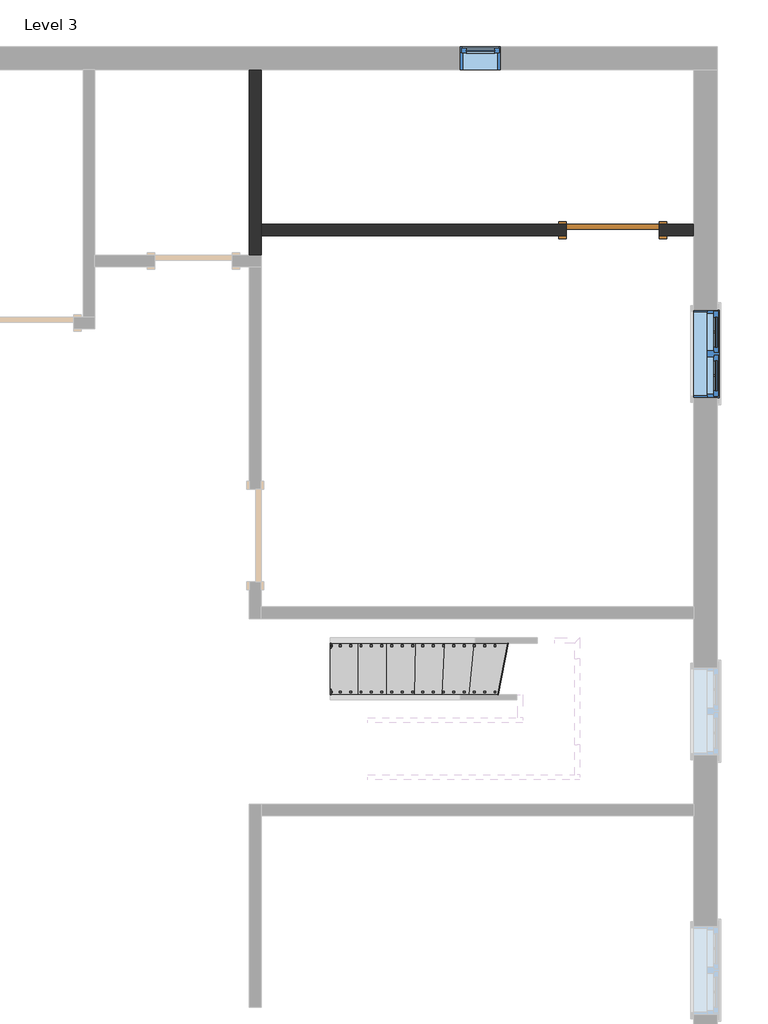
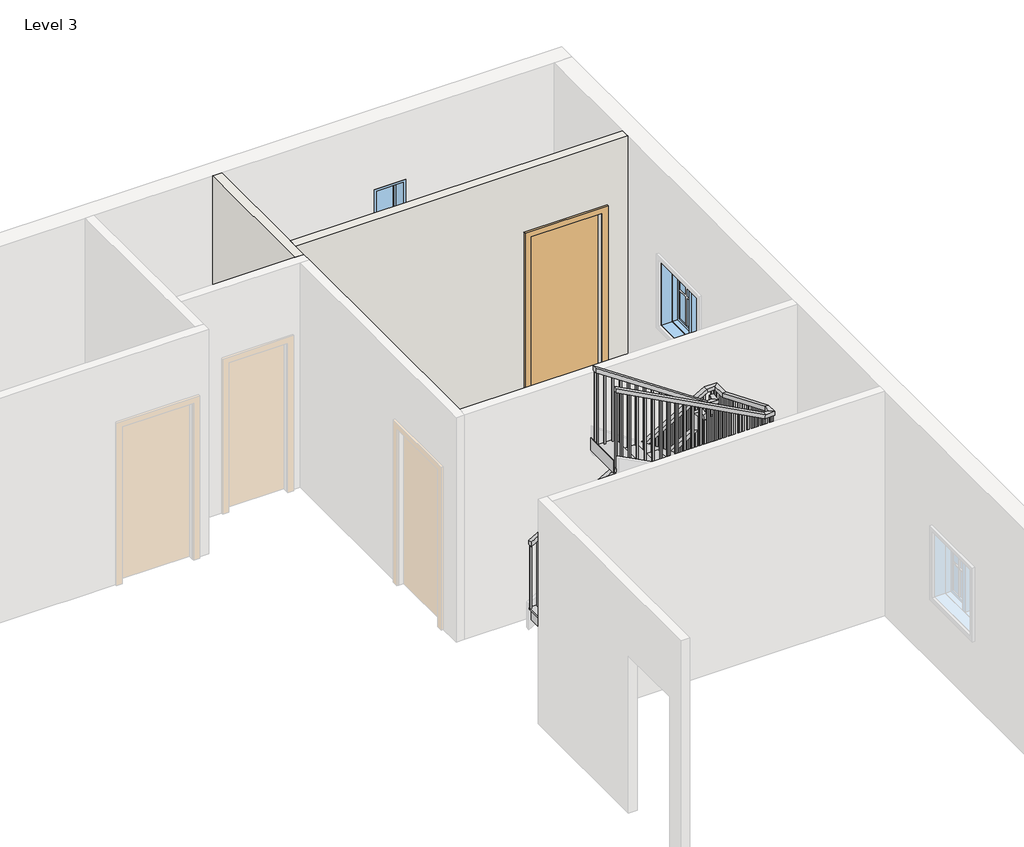
# One storey, part 2 of 3: 2 railings, 2 walls, 2 windows, 1 door, 1 stair flight.
"""IFC4 building model written with IfcOpenShell, lengths in millimetres."""

from ifc_helpers import new_model, si_unit, frame, origin, place, context, project, spatial, polyline, outline, extrude, faceted_brep, transform, mapped, element, save
from components import door_e5f9f3c4, stair_flight_4e66bfb9, window_373d1f99, window_339605e1

model = new_model("IFC4")

# Units and contexts
model_context = context("Model", 3, world=origin())
ifc_project = project(units=[si_unit("LENGTHUNIT", "METRE", prefix="MILLI")], contexts=[model_context])

# Site, building, storey
site = spatial("IfcSite", under=ifc_project)
building = spatial("IfcBuilding", under=site)
storey = spatial("IfcBuildingStorey", under=building, Name="Level 3", Elevation=3200.4)

# Door
placement = place(None, origin())
door_shape = door_e5f9f3c4(model_context)
element("IfcDoor", 1, ObjectType="Single-Flush : 36\" x 84\"", at=placement, inside=storey, context=model_context, shape_type="MappedRepresentation", body=[
    mapped(door_shape, transform((3624.6756993, 7272.227558, 3200.4), x_axis=(1.0, 0.0, 0.0), y_axis=(0.0, 1.0, 0.0), z_axis=(0.0, 0.0, 1.0))),
])

# Railings
element("IfcRailing", 2, ObjectType="Handrail - Rectangular", at=placement, inside=storey, context=model_context, shape_type="SolidModel", body=[
    faceted_brep([(838.4202681, 2744.677558, 4453.4666667), (838.4202681, 2744.677558, 4393.1442501), (838.4202681, 2693.877558, 4393.1442501), (838.4202681, 2693.877558, 4453.4666667), (2663.2073911, 2744.677558, 5621.9510761), (2714.0073911, 2744.677558, 5594.1579377), (2714.0073911, 2693.877558, 5594.1579377), (2663.2073911, 2693.877558, 5621.9510761), (2663.2073911, 2744.677558, 5834.2070819), (2714.0073911, 2744.677558, 5783.4070819), (2714.0073911, 2693.877558, 5783.4070819), (2663.2073911, 2693.877558, 5834.2070819), (2790.2073911, 2744.677558, 5834.2070819), (2790.2073911, 2744.677558, 5783.4070819), (2739.4073911, 2693.877558, 5783.4070819), (2739.4073911, 2693.877558, 5834.2070819), (2790.2073911, 2617.677558, 5834.2070819), (2790.2073911, 2595.5706127, 5783.4070819), (2739.4073911, 2595.5706127, 5783.4070819), (2739.4073911, 2617.677558, 5834.2070819), (2790.2073911, 2490.677558, 5970.5650362), (2790.2073911, 2439.877558, 5950.5723294), (2739.4073911, 2439.877558, 5950.5723294), (2739.4073911, 2490.677558, 5970.5650362), (2790.2073911, 2490.677558, 6186.1137911), (2790.2073911, 2439.877558, 6135.3137911), (2739.4073911, 2439.877558, 6135.3137911), (2739.4073911, 2490.677558, 6186.1137911), (2790.2073911, 2363.677558, 6186.1137911), (2790.2073911, 2363.677558, 6135.3137911), (2739.4073911, 2414.477558, 6135.3137911), (2739.4073911, 2414.477558, 6186.1137911), (2663.2073911, 2363.677558, 6186.1137911), (2647.7076469, 2363.677558, 6135.3137911), (2647.7076469, 2414.477558, 6135.3137911), (2663.2073911, 2414.477558, 6186.1137911), (1211.6756993, 2363.677558, 7162.8), (1211.6756993, 2414.477558, 7162.8), (1211.6756993, 2414.477558, 7101.5707504), (1211.6756993, 2363.677558, 7101.5707504)], [[[0, 1, 2, 3]], [[1, 0, 4, 5]], [[2, 1, 5, 6]], [[3, 2, 6, 7]], [[0, 3, 7, 4]], [[5, 4, 8, 9]], [[6, 5, 9, 10]], [[7, 6, 10, 11]], [[4, 7, 11, 8]], [[9, 8, 12, 13]], [[10, 9, 13, 14]], [[11, 10, 14, 15]], [[8, 11, 15, 12]], [[13, 12, 16, 17]], [[14, 13, 17, 18]], [[15, 14, 18, 19]], [[12, 15, 19, 16]], [[17, 16, 20, 21]], [[18, 17, 21, 22]], [[19, 18, 22, 23]], [[16, 19, 23, 20]], [[21, 20, 24, 25]], [[22, 21, 25, 26]], [[23, 22, 26, 27]], [[20, 23, 27, 24]], [[25, 24, 28, 29]], [[26, 25, 29, 30]], [[27, 26, 30, 31]], [[24, 27, 31, 28]], [[29, 28, 32, 33]], [[30, 29, 33, 34]], [[31, 30, 34, 35]], [[28, 31, 35, 32]], [[36, 37, 38, 39]], [[33, 32, 36, 39]], [[34, 33, 39, 38]], [[35, 34, 38, 37]], [[32, 35, 37, 36]]]),
    extrude(outline(polyline([(7075.5599798, 1250.3323911), (7088.3780756, 1231.2823911), (6079.0666667, 1231.2823911), (6079.0666667, 1250.3323911), (7075.5599798, 1250.3323911)])), frame((0.0, 2379.552558, 0.0), z_axis=(0.0, 1.0, 0.0), x_axis=(0.0, 0.0, 1.0)), (0.0, 0.0, 1.0), 19.05),
    extrude(outline(polyline([(7007.1968022, 1351.9323911), (7020.014898, 1332.8823911), (6079.0666667, 1332.8823911), (6079.0666667, 1351.9323911), (7007.1968022, 1351.9323911)])), frame((0.0, 2379.552558, 0.0), z_axis=(0.0, 1.0, 0.0), x_axis=(0.0, 0.0, 1.0)), (0.0, 0.0, 1.0), 19.05),
    extrude(outline(polyline([(6938.8336246, 1453.5323911), (6951.6517204, 1434.4823911), (6079.0666667, 1434.4823911), (6079.0666667, 1453.5323911), (6938.8336246, 1453.5323911)])), frame((0.0, 2379.552558, 0.0), z_axis=(0.0, 1.0, 0.0), x_axis=(0.0, 0.0, 1.0)), (0.0, 0.0, 1.0), 19.05),
    extrude(outline(polyline([(6870.470447, 1555.1323911), (6883.2885428, 1536.0823911), (5909.7333333, 1536.0823911), (5909.7333333, 1555.1323911), (6870.470447, 1555.1323911)])), frame((0.0, 2379.552558, 0.0), z_axis=(0.0, 1.0, 0.0), x_axis=(0.0, 0.0, 1.0)), (0.0, 0.0, 1.0), 19.05),
    extrude(outline(polyline([(6802.1072694, 1656.7323911), (6814.9253652, 1637.6823911), (5909.7333333, 1637.6823911), (5909.7333333, 1656.7323911), (6802.1072694, 1656.7323911)])), frame((0.0, 2379.552558, 0.0), z_axis=(0.0, 1.0, 0.0), x_axis=(0.0, 0.0, 1.0)), (0.0, 0.0, 1.0), 19.05),
    extrude(outline(polyline([(6733.7440918, 1758.3323911), (6746.5621876, 1739.2823911), (5909.7333333, 1739.2823911), (5909.7333333, 1758.3323911), (6733.7440918, 1758.3323911)])), frame((0.0, 2379.552558, 0.0), z_axis=(0.0, 1.0, 0.0), x_axis=(0.0, 0.0, 1.0)), (0.0, 0.0, 1.0), 19.05),
    extrude(outline(polyline([(6665.3809143, 1859.9323911), (6678.1990101, 1840.8823911), (5740.4, 1840.8823911), (5740.4, 1859.9323911), (6665.3809143, 1859.9323911)])), frame((0.0, 2379.552558, 0.0), z_axis=(0.0, 1.0, 0.0), x_axis=(0.0, 0.0, 1.0)), (0.0, 0.0, 1.0), 19.05),
    extrude(outline(polyline([(6597.0177367, 1961.5323911), (6609.8358325, 1942.4823911), (5740.4, 1942.4823911), (5740.4, 1961.5323911), (6597.0177367, 1961.5323911)])), frame((0.0, 2379.552558, 0.0), z_axis=(0.0, 1.0, 0.0), x_axis=(0.0, 0.0, 1.0)), (0.0, 0.0, 1.0), 19.05),
    extrude(outline(polyline([(6528.6545591, 2063.1323911), (6541.4726549, 2044.0823911), (5571.0666667, 2044.0823911), (5571.0666667, 2063.1323911), (6528.6545591, 2063.1323911)])), frame((0.0, 2379.552558, 0.0), z_axis=(0.0, 1.0, 0.0), x_axis=(0.0, 0.0, 1.0)), (0.0, 0.0, 1.0), 19.05),
    extrude(outline(polyline([(6460.2913815, 2164.7323911), (6473.1094773, 2145.6823911), (5571.0666667, 2145.6823911), (5571.0666667, 2164.7323911), (6460.2913815, 2164.7323911)])), frame((0.0, 2379.552558, 0.0), z_axis=(0.0, 1.0, 0.0), x_axis=(0.0, 0.0, 1.0)), (0.0, 0.0, 1.0), 19.05),
    extrude(outline(polyline([(6391.9282039, 2266.3323911), (6404.7462997, 2247.2823911), (5571.0666667, 2247.2823911), (5571.0666667, 2266.3323911), (6391.9282039, 2266.3323911)])), frame((0.0, 2379.552558, 0.0), z_axis=(0.0, 1.0, 0.0), x_axis=(0.0, 0.0, 1.0)), (0.0, 0.0, 1.0), 19.05),
    extrude(outline(polyline([(6323.5650263, 2367.9323911), (6336.3831221, 2348.8823911), (5401.7333333, 2348.8823911), (5401.7333333, 2367.9323911), (6323.5650263, 2367.9323911)])), frame((0.0, 2379.552558, 0.0), z_axis=(0.0, 1.0, 0.0), x_axis=(0.0, 0.0, 1.0)), (0.0, 0.0, 1.0), 19.05),
    extrude(outline(polyline([(6255.2018487, 2469.5323911), (6268.0199445, 2450.4823911), (5401.7333333, 2450.4823911), (5401.7333333, 2469.5323911), (6255.2018487, 2469.5323911)])), frame((0.0, 2379.552558, 0.0), z_axis=(0.0, 1.0, 0.0), x_axis=(0.0, 0.0, 1.0)), (0.0, 0.0, 1.0), 19.05),
    extrude(outline(polyline([(6186.8386712, 2571.1323911), (6199.656767, 2552.0823911), (5232.4, 2552.0823911), (5232.4, 2571.1323911), (6186.8386712, 2571.1323911)])), frame((0.0, 2379.552558, 0.0), z_axis=(0.0, 1.0, 0.0), x_axis=(0.0, 0.0, 1.0)), (0.0, 0.0, 1.0), 19.05),
    extrude(outline(polyline([(6118.4754936, 2672.7323911), (6131.2935894, 2653.6823911), (5232.4, 2653.6823911), (5232.4, 2672.7323911), (6118.4754936, 2672.7323911)])), frame((0.0, 2379.552558, 0.0), z_axis=(0.0, 1.0, 0.0), x_axis=(0.0, 0.0, 1.0)), (0.0, 0.0, 1.0), 19.05),
    extrude(outline(polyline([(2755.2823911, 2424.002558), (2774.3323911, 2424.002558), (2774.3323911, 2404.952558), (2755.2823911, 2404.952558), (2755.2823911, 2424.002558)])), frame((0.0, 0.0, 5063.0666667), z_axis=(0.0, 0.0, 1.0), x_axis=(1.0, 0.0, 0.0)), (0.0, 0.0, 1.0), 1072.2471245),
    extrude(outline(polyline([(2506.552558, 5878.9844034), (2525.602558, 5858.5307103), (2525.602558, 4893.7333333), (2506.552558, 4893.7333333), (2506.552558, 5878.9844034)])), frame((2755.2823911, 0.0, 0.0), z_axis=(1.0, 0.0, 0.0), x_axis=(0.0, 1.0, 0.0)), (0.0, 0.0, 1.0), 19.05),
    extrude(outline(polyline([(2608.152558, 5769.89804), (2627.202558, 5749.4443468), (2627.202558, 4893.7333333), (2608.152558, 4893.7333333), (2608.152558, 5769.89804)])), frame((2755.2823911, 0.0, 0.0), z_axis=(1.0, 0.0, 0.0), x_axis=(0.0, 1.0, 0.0)), (0.0, 0.0, 1.0), 19.05),
    extrude(outline(polyline([(2657.6952681, 2709.752558), (2657.6952681, 2728.802558), (2676.7452681, 2728.802558), (2676.7452681, 2709.752558), (2657.6952681, 2709.752558)])), frame((0.0, 0.0, 4555.0666667), z_axis=(0.0, 0.0, 1.0), x_axis=(1.0, 0.0, 0.0)), (0.0, 0.0, 1.0), 1228.3404152),
    extrude(outline(polyline([(5505.2389489, 2575.1452681), (5493.0404695, 2556.0952681), (4555.0666667, 2556.0952681), (4555.0666667, 2575.1452681), (5505.2389489, 2575.1452681)])), frame((0.0, 2709.752558, 0.0), z_axis=(0.0, 1.0, 0.0), x_axis=(0.0, 0.0, 1.0)), (0.0, 0.0, 1.0), 19.05),
    extrude(outline(polyline([(5440.1803925, 2473.5452681), (5427.9819131, 2454.4952681), (4385.7333333, 2454.4952681), (4385.7333333, 2473.5452681), (5440.1803925, 2473.5452681)])), frame((0.0, 2709.752558, 0.0), z_axis=(0.0, 1.0, 0.0), x_axis=(0.0, 0.0, 1.0)), (0.0, 0.0, 1.0), 19.05),
    extrude(outline(polyline([(5375.121836, 2371.9452681), (5362.9233567, 2352.8952681), (4385.7333333, 2352.8952681), (4385.7333333, 2371.9452681), (5375.121836, 2371.9452681)])), frame((0.0, 2709.752558, 0.0), z_axis=(0.0, 1.0, 0.0), x_axis=(0.0, 0.0, 1.0)), (0.0, 0.0, 1.0), 19.05),
    extrude(outline(polyline([(5310.0632796, 2270.3452681), (5297.8648003, 2251.2952681), (4385.7333333, 2251.2952681), (4385.7333333, 2270.3452681), (5310.0632796, 2270.3452681)])), frame((0.0, 2709.752558, 0.0), z_axis=(0.0, 1.0, 0.0), x_axis=(0.0, 0.0, 1.0)), (0.0, 0.0, 1.0), 19.05),
    extrude(outline(polyline([(5245.0047232, 2168.7452681), (5232.8062439, 2149.6952681), (4216.4, 2149.6952681), (4216.4, 2168.7452681), (5245.0047232, 2168.7452681)])), frame((0.0, 2709.752558, 0.0), z_axis=(0.0, 1.0, 0.0), x_axis=(0.0, 0.0, 1.0)), (0.0, 0.0, 1.0), 19.05),
    extrude(outline(polyline([(5179.9461668, 2067.1452681), (5167.7476875, 2048.0952681), (4216.4, 2048.0952681), (4216.4, 2067.1452681), (5179.9461668, 2067.1452681)])), frame((0.0, 2709.752558, 0.0), z_axis=(0.0, 1.0, 0.0), x_axis=(0.0, 0.0, 1.0)), (0.0, 0.0, 1.0), 19.05),
    extrude(outline(polyline([(5114.8876104, 1965.5452681), (5102.689131, 1946.4952681), (4216.4, 1946.4952681), (4216.4, 1965.5452681), (5114.8876104, 1965.5452681)])), frame((0.0, 2709.752558, 0.0), z_axis=(0.0, 1.0, 0.0), x_axis=(0.0, 0.0, 1.0)), (0.0, 0.0, 1.0), 19.05),
    extrude(outline(polyline([(5049.8290539, 1863.9452681), (5037.6305746, 1844.8952681), (4047.0666667, 1844.8952681), (4047.0666667, 1863.9452681), (5049.8290539, 1863.9452681)])), frame((0.0, 2709.752558, 0.0), z_axis=(0.0, 1.0, 0.0), x_axis=(0.0, 0.0, 1.0)), (0.0, 0.0, 1.0), 19.05),
    extrude(outline(polyline([(4984.7704975, 1762.3452681), (4972.5720182, 1743.2952681), (4047.0666667, 1743.2952681), (4047.0666667, 1762.3452681), (4984.7704975, 1762.3452681)])), frame((0.0, 2709.752558, 0.0), z_axis=(0.0, 1.0, 0.0), x_axis=(0.0, 0.0, 1.0)), (0.0, 0.0, 1.0), 19.05),
    extrude(outline(polyline([(4919.7119411, 1660.7452681), (4907.5134618, 1641.6952681), (3877.7333333, 1641.6952681), (3877.7333333, 1660.7452681), (4919.7119411, 1660.7452681)])), frame((0.0, 2709.752558, 0.0), z_axis=(0.0, 1.0, 0.0), x_axis=(0.0, 0.0, 1.0)), (0.0, 0.0, 1.0), 19.05),
    extrude(outline(polyline([(4854.6533847, 1559.1452681), (4842.4549054, 1540.0952681), (3877.7333333, 1540.0952681), (3877.7333333, 1559.1452681), (4854.6533847, 1559.1452681)])), frame((0.0, 2709.752558, 0.0), z_axis=(0.0, 1.0, 0.0), x_axis=(0.0, 0.0, 1.0)), (0.0, 0.0, 1.0), 19.05),
    extrude(outline(polyline([(4789.5948283, 1457.5452681), (4777.3963489, 1438.4952681), (3877.7333333, 1438.4952681), (3877.7333333, 1457.5452681), (4789.5948283, 1457.5452681)])), frame((0.0, 2709.752558, 0.0), z_axis=(0.0, 1.0, 0.0), x_axis=(0.0, 0.0, 1.0)), (0.0, 0.0, 1.0), 19.05),
    extrude(outline(polyline([(4724.5362719, 1355.9452681), (4712.3377925, 1336.8952681), (3708.4, 1336.8952681), (3708.4, 1355.9452681), (4724.5362719, 1355.9452681)])), frame((0.0, 2709.752558, 0.0), z_axis=(0.0, 1.0, 0.0), x_axis=(0.0, 0.0, 1.0)), (0.0, 0.0, 1.0), 19.05),
    extrude(outline(polyline([(4659.4777154, 1254.3452681), (4647.2792361, 1235.2952681), (3708.4, 1235.2952681), (3708.4, 1254.3452681), (4659.4777154, 1254.3452681)])), frame((0.0, 2709.752558, 0.0), z_axis=(0.0, 1.0, 0.0), x_axis=(0.0, 0.0, 1.0)), (0.0, 0.0, 1.0), 19.05),
    extrude(outline(polyline([(4594.419159, 1152.7452681), (4582.2206797, 1133.6952681), (3708.4, 1133.6952681), (3708.4, 1152.7452681), (4594.419159, 1152.7452681)])), frame((0.0, 2709.752558, 0.0), z_axis=(0.0, 1.0, 0.0), x_axis=(0.0, 0.0, 1.0)), (0.0, 0.0, 1.0), 19.05),
    extrude(outline(polyline([(4529.3606026, 1051.1452681), (4517.1621233, 1032.0952681), (3539.0666667, 1032.0952681), (3539.0666667, 1051.1452681), (4529.3606026, 1051.1452681)])), frame((0.0, 2709.752558, 0.0), z_axis=(0.0, 1.0, 0.0), x_axis=(0.0, 0.0, 1.0)), (0.0, 0.0, 1.0), 19.05),
    extrude(outline(polyline([(4464.3020462, 949.5452681), (4452.1035669, 930.4952681), (3539.0666667, 930.4952681), (3539.0666667, 949.5452681), (4464.3020462, 949.5452681)])), frame((0.0, 2709.752558, 0.0), z_axis=(0.0, 1.0, 0.0), x_axis=(0.0, 0.0, 1.0)), (0.0, 0.0, 1.0), 19.05),
    extrude(outline(polyline([(2755.2823911, 2398.602558), (2774.3323911, 2398.602558), (2774.3323911, 2379.552558), (2755.2823911, 2379.552558), (2755.2823911, 2398.602558)])), frame((0.0, 0.0, 5063.0666667), z_axis=(0.0, 0.0, 1.0), x_axis=(1.0, 0.0, 0.0)), (0.0, 0.0, 1.0), 1072.2471245),
    extrude(outline(polyline([(2755.2823911, 2709.752558), (2755.2823911, 2728.802558), (2774.3323911, 2728.802558), (2774.3323911, 2709.752558), (2755.2823911, 2709.752558)])), frame((0.0, 0.0, 4724.4), z_axis=(0.0, 0.0, 1.0), x_axis=(1.0, 0.0, 0.0)), (0.0, 0.0, 1.0), 1059.0070819),
    extrude(outline(polyline([(7088.7526546, 1230.7256993), (7101.5707504, 1211.6756993), (6079.0666667, 1211.6756993), (6079.0666667, 1230.7256993), (7088.7526546, 1230.7256993)])), frame((0.0, 2379.552558, 0.0), z_axis=(0.0, 1.0, 0.0), x_axis=(0.0, 0.0, 1.0)), (0.0, 0.0, 1.0), 19.05),
    extrude(outline(polyline([(4405.3427294, 857.4702681), (4393.1442501, 838.4202681), (3539.0666667, 838.4202681), (3539.0666667, 857.4702681), (4405.3427294, 857.4702681)])), frame((0.0, 2709.752558, 0.0), z_axis=(0.0, 1.0, 0.0), x_axis=(0.0, 0.0, 1.0)), (0.0, 0.0, 1.0), 19.05),
])
element("IfcRailing", 3, ObjectType="Handrail - Rectangular", at=placement, inside=storey, context=model_context, shape_type="SolidModel", body=[
    faceted_brep([(838.4202681, 3202.4524989, 4453.4666667), (838.4202681, 3202.4524989, 4394.8953096), (838.4202681, 3151.6524989, 4394.8953096), (838.4202681, 3151.6524989, 4453.4666667), (3089.9785641, 3202.4524989, 5745.6368493), (3103.5198636, 3202.4524989, 5694.8368493), (3103.5198636, 3151.6524989, 5694.8368493), (3089.9785641, 3151.6524989, 5745.6368493), (3247.982332, 3202.4524989, 5745.6368493), (3247.982332, 3202.4524989, 5694.8368493), (3197.182332, 3151.6524989, 5694.8368493), (3197.182332, 3151.6524989, 5745.6368493), (3247.982332, 2995.1725832, 5745.6368493), (3247.982332, 2984.9732412, 5694.8368493), (3197.182332, 2984.9732412, 5694.8368493), (3197.182332, 2995.1725832, 5745.6368493), (3247.982332, 2050.6126885, 6140.8552365), (3247.982332, 2040.4133465, 6090.0552365), (3197.182332, 2040.4133465, 6090.0552365), (3197.182332, 2050.6126885, 6140.8552365), (3247.982332, 1905.9026171, 6140.8552365), (3247.982332, 1905.9026171, 6090.0552365), (3197.182332, 1956.7026171, 6090.0552365), (3197.182332, 1956.7026171, 6140.8552365), (3128.9262072, 1905.9026171, 6140.8552365), (3116.2326609, 1905.9026171, 6090.0552365), (3116.2326609, 1956.7026171, 6090.0552365), (3128.9262072, 1956.7026171, 6140.8552365), (1211.6756993, 1905.9026171, 7162.8), (1211.6756993, 1956.7026171, 7162.8), (1211.6756993, 1956.7026171, 7105.2340072), (1211.6756993, 1905.9026171, 7105.2340072)], [[[0, 1, 2, 3]], [[1, 0, 4, 5]], [[2, 1, 5, 6]], [[3, 2, 6, 7]], [[0, 3, 7, 4]], [[5, 4, 8, 9]], [[6, 5, 9, 10]], [[7, 6, 10, 11]], [[4, 7, 11, 8]], [[9, 8, 12, 13]], [[10, 9, 13, 14]], [[11, 10, 14, 15]], [[8, 11, 15, 12]], [[13, 12, 16, 17]], [[14, 13, 17, 18]], [[15, 14, 18, 19]], [[12, 15, 19, 16]], [[17, 16, 20, 21]], [[18, 17, 21, 22]], [[19, 18, 22, 23]], [[16, 19, 23, 20]], [[21, 20, 24, 25]], [[22, 21, 25, 26]], [[23, 22, 26, 27]], [[20, 23, 27, 24]], [[28, 29, 30, 31]], [[25, 24, 28, 31]], [[26, 25, 31, 30]], [[27, 26, 30, 29]], [[24, 27, 29, 28]]]),
    extrude(outline(polyline([(7067.3989368, 1282.657332), (6079.0666667, 1282.657332), (6079.0666667, 1301.707332), (7057.2447876, 1301.707332), (7067.3989368, 1282.657332)])), frame((0.0, 1921.7776171, 0.0), z_axis=(0.0, 1.0, 0.0), x_axis=(0.0, 0.0, 1.0)), (0.0, 0.0, 1.0), 19.05),
    extrude(outline(polyline([(7013.2434743, 1384.257332), (6079.0666667, 1384.257332), (6079.0666667, 1403.307332), (7003.0893251, 1403.307332), (7013.2434743, 1384.257332)])), frame((0.0, 1921.7776171, 0.0), z_axis=(0.0, 1.0, 0.0), x_axis=(0.0, 0.0, 1.0)), (0.0, 0.0, 1.0), 19.05),
    extrude(outline(polyline([(6959.0880118, 1485.857332), (5909.7333333, 1485.857332), (5909.7333333, 1504.907332), (6948.9338626, 1504.907332), (6959.0880118, 1485.857332)])), frame((0.0, 1921.7776171, 0.0), z_axis=(0.0, 1.0, 0.0), x_axis=(0.0, 0.0, 1.0)), (0.0, 0.0, 1.0), 19.05),
    extrude(outline(polyline([(6904.9325493, 1587.457332), (5909.7333333, 1587.457332), (5909.7333333, 1606.507332), (6894.7784001, 1606.507332), (6904.9325493, 1587.457332)])), frame((0.0, 1921.7776171, 0.0), z_axis=(0.0, 1.0, 0.0), x_axis=(0.0, 0.0, 1.0)), (0.0, 0.0, 1.0), 19.05),
    extrude(outline(polyline([(6850.7770868, 1689.057332), (5909.7333333, 1689.057332), (5909.7333333, 1708.107332), (6840.6229376, 1708.107332), (6850.7770868, 1689.057332)])), frame((0.0, 1921.7776171, 0.0), z_axis=(0.0, 1.0, 0.0), x_axis=(0.0, 0.0, 1.0)), (0.0, 0.0, 1.0), 19.05),
    extrude(outline(polyline([(6796.6216243, 1790.657332), (5740.4, 1790.657332), (5740.4, 1809.707332), (6786.4674751, 1809.707332), (6796.6216243, 1790.657332)])), frame((0.0, 1921.7776171, 0.0), z_axis=(0.0, 1.0, 0.0), x_axis=(0.0, 0.0, 1.0)), (0.0, 0.0, 1.0), 19.05),
    extrude(outline(polyline([(6742.4661618, 1892.257332), (5740.4, 1892.257332), (5740.4, 1911.307332), (6732.3120126, 1911.307332), (6742.4661618, 1892.257332)])), frame((0.0, 1921.7776171, 0.0), z_axis=(0.0, 1.0, 0.0), x_axis=(0.0, 0.0, 1.0)), (0.0, 0.0, 1.0), 19.05),
    extrude(outline(polyline([(6688.3106993, 1993.857332), (5740.4, 1993.857332), (5740.4, 2012.907332), (6678.1565501, 2012.907332), (6688.3106993, 1993.857332)])), frame((0.0, 1921.7776171, 0.0), z_axis=(0.0, 1.0, 0.0), x_axis=(0.0, 0.0, 1.0)), (0.0, 0.0, 1.0), 19.05),
    extrude(outline(polyline([(6634.1552369, 2095.457332), (5571.0666667, 2095.457332), (5571.0666667, 2114.507332), (6624.0010876, 2114.507332), (6634.1552369, 2095.457332)])), frame((0.0, 1921.7776171, 0.0), z_axis=(0.0, 1.0, 0.0), x_axis=(0.0, 0.0, 1.0)), (0.0, 0.0, 1.0), 19.05),
    extrude(outline(polyline([(6579.9997744, 2197.057332), (5571.0666667, 2197.057332), (5571.0666667, 2216.107332), (6569.8456251, 2216.107332), (6579.9997744, 2197.057332)])), frame((0.0, 1921.7776171, 0.0), z_axis=(0.0, 1.0, 0.0), x_axis=(0.0, 0.0, 1.0)), (0.0, 0.0, 1.0), 19.05),
    extrude(outline(polyline([(6525.8443119, 2298.657332), (5571.0666667, 2298.657332), (5571.0666667, 2317.707332), (6515.6901626, 2317.707332), (6525.8443119, 2298.657332)])), frame((0.0, 1921.7776171, 0.0), z_axis=(0.0, 1.0, 0.0), x_axis=(0.0, 0.0, 1.0)), (0.0, 0.0, 1.0), 19.05),
    extrude(outline(polyline([(6471.6888494, 2400.257332), (5401.7333333, 2400.257332), (5401.7333333, 2419.307332), (6461.5347002, 2419.307332), (6471.6888494, 2400.257332)])), frame((0.0, 1921.7776171, 0.0), z_axis=(0.0, 1.0, 0.0), x_axis=(0.0, 0.0, 1.0)), (0.0, 0.0, 1.0), 19.05),
    extrude(outline(polyline([(6417.5333869, 2501.857332), (5401.7333333, 2501.857332), (5401.7333333, 2520.907332), (6407.3792377, 2520.907332), (6417.5333869, 2501.857332)])), frame((0.0, 1921.7776171, 0.0), z_axis=(0.0, 1.0, 0.0), x_axis=(0.0, 0.0, 1.0)), (0.0, 0.0, 1.0), 19.05),
    extrude(outline(polyline([(6363.3779244, 2603.457332), (5401.7333333, 2603.457332), (5401.7333333, 2622.507332), (6353.2237752, 2622.507332), (6363.3779244, 2603.457332)])), frame((0.0, 1921.7776171, 0.0), z_axis=(0.0, 1.0, 0.0), x_axis=(0.0, 0.0, 1.0)), (0.0, 0.0, 1.0), 19.05),
    extrude(outline(polyline([(6309.2224619, 2705.057332), (5232.4, 2705.057332), (5232.4, 2724.107332), (6299.0683127, 2724.107332), (6309.2224619, 2705.057332)])), frame((0.0, 1921.7776171, 0.0), z_axis=(0.0, 1.0, 0.0), x_axis=(0.0, 0.0, 1.0)), (0.0, 0.0, 1.0), 19.05),
    extrude(outline(polyline([(6255.0669994, 2806.657332), (5232.4, 2806.657332), (5232.4, 2825.707332), (6244.9128502, 2825.707332), (6255.0669994, 2806.657332)])), frame((0.0, 1921.7776171, 0.0), z_axis=(0.0, 1.0, 0.0), x_axis=(0.0, 0.0, 1.0)), (0.0, 0.0, 1.0), 19.05),
    extrude(outline(polyline([(6200.9115369, 2908.257332), (5232.4, 2908.257332), (5232.4, 2927.307332), (6190.7573877, 2927.307332), (6200.9115369, 2908.257332)])), frame((0.0, 1921.7776171, 0.0), z_axis=(0.0, 1.0, 0.0), x_axis=(0.0, 0.0, 1.0)), (0.0, 0.0, 1.0), 19.05),
    extrude(outline(polyline([(6146.7560744, 3009.857332), (5232.4, 3009.857332), (5232.4, 3028.907332), (6136.6019252, 3028.907332), (6146.7560744, 3009.857332)])), frame((0.0, 1921.7776171, 0.0), z_axis=(0.0, 1.0, 0.0), x_axis=(0.0, 0.0, 1.0)), (0.0, 0.0, 1.0), 19.05),
    extrude(outline(polyline([(6092.6006119, 3111.457332), (5063.0666667, 3111.457332), (5063.0666667, 3130.507332), (6082.4464627, 3130.507332), (6092.6006119, 3111.457332)])), frame((0.0, 1921.7776171, 0.0), z_axis=(0.0, 1.0, 0.0), x_axis=(0.0, 0.0, 1.0)), (0.0, 0.0, 1.0), 19.05),
    extrude(outline(polyline([(3232.107332, 1967.3774989), (3232.107332, 1948.3274989), (3213.057332, 1948.3274989), (3213.057332, 1967.3774989), (3232.107332, 1967.3774989)])), frame((0.0, 0.0, 5063.0666667), z_axis=(0.0, 0.0, 1.0), x_axis=(1.0, 0.0, 0.0)), (0.0, 0.0, 1.0), 1026.9885698),
    extrude(outline(polyline([(2068.9774989, 6078.1035558), (2068.9774989, 5063.0666667), (2049.9274989, 5063.0666667), (2049.9274989, 6086.0743688), (2068.9774989, 6078.1035558)])), frame((3213.057332, 0.0, 0.0), z_axis=(1.0, 0.0, 0.0), x_axis=(0.0, 1.0, 0.0)), (0.0, 0.0, 1.0), 19.05),
    extrude(outline(polyline([(2170.5774989, 6035.5925532), (2170.5774989, 5063.0666667), (2151.5274989, 5063.0666667), (2151.5274989, 6043.5633662), (2170.5774989, 6035.5925532)])), frame((3213.057332, 0.0, 0.0), z_axis=(1.0, 0.0, 0.0), x_axis=(0.0, 1.0, 0.0)), (0.0, 0.0, 1.0), 19.05),
    extrude(outline(polyline([(2272.1774989, 5993.0815506), (2272.1774989, 5063.0666667), (2253.1274989, 5063.0666667), (2253.1274989, 6001.0523636), (2272.1774989, 5993.0815506)])), frame((3213.057332, 0.0, 0.0), z_axis=(1.0, 0.0, 0.0), x_axis=(0.0, 1.0, 0.0)), (0.0, 0.0, 1.0), 19.05),
    extrude(outline(polyline([(2373.7774989, 5950.570548), (2373.7774989, 5063.0666667), (2354.7274989, 5063.0666667), (2354.7274989, 5958.541361), (2373.7774989, 5950.570548)])), frame((3213.057332, 0.0, 0.0), z_axis=(1.0, 0.0, 0.0), x_axis=(0.0, 1.0, 0.0)), (0.0, 0.0, 1.0), 19.05),
    extrude(outline(polyline([(2475.3774989, 5908.0595454), (2475.3774989, 4893.7333333), (2456.3274989, 4893.7333333), (2456.3274989, 5916.0303584), (2475.3774989, 5908.0595454)])), frame((3213.057332, 0.0, 0.0), z_axis=(1.0, 0.0, 0.0), x_axis=(0.0, 1.0, 0.0)), (0.0, 0.0, 1.0), 19.05),
    extrude(outline(polyline([(2576.9774989, 5865.5485428), (2576.9774989, 4893.7333333), (2557.9274989, 4893.7333333), (2557.9274989, 5873.5193558), (2576.9774989, 5865.5485428)])), frame((3213.057332, 0.0, 0.0), z_axis=(1.0, 0.0, 0.0), x_axis=(0.0, 1.0, 0.0)), (0.0, 0.0, 1.0), 19.05),
    extrude(outline(polyline([(2678.5774989, 5823.0375402), (2678.5774989, 4893.7333333), (2659.5274989, 4893.7333333), (2659.5274989, 5831.0083532), (2678.5774989, 5823.0375402)])), frame((3213.057332, 0.0, 0.0), z_axis=(1.0, 0.0, 0.0), x_axis=(0.0, 1.0, 0.0)), (0.0, 0.0, 1.0), 19.05),
    extrude(outline(polyline([(2780.1774989, 5780.5265376), (2780.1774989, 4893.7333333), (2761.1274989, 4893.7333333), (2761.1274989, 5788.4973506), (2780.1774989, 5780.5265376)])), frame((3213.057332, 0.0, 0.0), z_axis=(1.0, 0.0, 0.0), x_axis=(0.0, 1.0, 0.0)), (0.0, 0.0, 1.0), 19.05),
    extrude(outline(polyline([(2881.7774989, 5738.015535), (2881.7774989, 4724.4), (2862.7274989, 4724.4), (2862.7274989, 5745.986348), (2881.7774989, 5738.015535)])), frame((3213.057332, 0.0, 0.0), z_axis=(1.0, 0.0, 0.0), x_axis=(0.0, 1.0, 0.0)), (0.0, 0.0, 1.0), 19.05),
    extrude(outline(polyline([(2983.3774989, 5695.5045324), (2983.3774989, 4724.4), (2964.3274989, 4724.4), (2964.3274989, 5703.4753454), (2983.3774989, 5695.5045324)])), frame((3213.057332, 0.0, 0.0), z_axis=(1.0, 0.0, 0.0), x_axis=(0.0, 1.0, 0.0)), (0.0, 0.0, 1.0), 19.05),
    extrude(outline(polyline([(3232.107332, 3084.9774989), (3232.107332, 3065.9274989), (3213.057332, 3065.9274989), (3213.057332, 3084.9774989), (3232.107332, 3084.9774989)])), frame((0.0, 0.0, 4724.4), z_axis=(0.0, 0.0, 1.0), x_axis=(1.0, 0.0, 0.0)), (0.0, 0.0, 1.0), 970.4368493),
    extrude(outline(polyline([(3165.6952681, 3186.5774989), (3184.7452681, 3186.5774989), (3184.7452681, 3167.5274989), (3165.6952681, 3167.5274989), (3165.6952681, 3186.5774989)])), frame((0.0, 0.0, 4724.4), z_axis=(0.0, 0.0, 1.0), x_axis=(1.0, 0.0, 0.0)), (0.0, 0.0, 1.0), 970.4368493),
    extrude(outline(polyline([(5672.2110585, 3064.0952681), (4724.4, 3064.0952681), (4724.4, 3083.1452681), (5683.143861, 3083.1452681), (5672.2110585, 3064.0952681)])), frame((0.0, 3167.5274989, 0.0), z_axis=(0.0, 1.0, 0.0), x_axis=(0.0, 0.0, 1.0)), (0.0, 0.0, 1.0), 19.05),
    extrude(outline(polyline([(5613.902779, 2962.4952681), (4724.4, 2962.4952681), (4724.4, 2981.5452681), (5624.8355814, 2981.5452681), (5613.902779, 2962.4952681)])), frame((0.0, 3167.5274989, 0.0), z_axis=(0.0, 1.0, 0.0), x_axis=(0.0, 0.0, 1.0)), (0.0, 0.0, 1.0), 19.05),
    extrude(outline(polyline([(5555.5944994, 2860.8952681), (4555.0666667, 2860.8952681), (4555.0666667, 2879.9452681), (5566.5273019, 2879.9452681), (5555.5944994, 2860.8952681)])), frame((0.0, 3167.5274989, 0.0), z_axis=(0.0, 1.0, 0.0), x_axis=(0.0, 0.0, 1.0)), (0.0, 0.0, 1.0), 19.05),
    extrude(outline(polyline([(5497.2862199, 2759.2952681), (4555.0666667, 2759.2952681), (4555.0666667, 2778.3452681), (5508.2190223, 2778.3452681), (5497.2862199, 2759.2952681)])), frame((0.0, 3167.5274989, 0.0), z_axis=(0.0, 1.0, 0.0), x_axis=(0.0, 0.0, 1.0)), (0.0, 0.0, 1.0), 19.05),
    extrude(outline(polyline([(5438.9779403, 2657.6952681), (4555.0666667, 2657.6952681), (4555.0666667, 2676.7452681), (5449.9107428, 2676.7452681), (5438.9779403, 2657.6952681)])), frame((0.0, 3167.5274989, 0.0), z_axis=(0.0, 1.0, 0.0), x_axis=(0.0, 0.0, 1.0)), (0.0, 0.0, 1.0), 19.05),
    extrude(outline(polyline([(5380.6696608, 2556.0952681), (4555.0666667, 2556.0952681), (4555.0666667, 2575.1452681), (5391.6024632, 2575.1452681), (5380.6696608, 2556.0952681)])), frame((0.0, 3167.5274989, 0.0), z_axis=(0.0, 1.0, 0.0), x_axis=(0.0, 0.0, 1.0)), (0.0, 0.0, 1.0), 19.05),
    extrude(outline(polyline([(5322.3613812, 2454.4952681), (4385.7333333, 2454.4952681), (4385.7333333, 2473.5452681), (5333.2941837, 2473.5452681), (5322.3613812, 2454.4952681)])), frame((0.0, 3167.5274989, 0.0), z_axis=(0.0, 1.0, 0.0), x_axis=(0.0, 0.0, 1.0)), (0.0, 0.0, 1.0), 19.05),
    extrude(outline(polyline([(5264.0531017, 2352.8952681), (4385.7333333, 2352.8952681), (4385.7333333, 2371.9452681), (5274.9859041, 2371.9452681), (5264.0531017, 2352.8952681)])), frame((0.0, 3167.5274989, 0.0), z_axis=(0.0, 1.0, 0.0), x_axis=(0.0, 0.0, 1.0)), (0.0, 0.0, 1.0), 19.05),
    extrude(outline(polyline([(5205.7448221, 2251.2952681), (4385.7333333, 2251.2952681), (4385.7333333, 2270.3452681), (5216.6776245, 2270.3452681), (5205.7448221, 2251.2952681)])), frame((0.0, 3167.5274989, 0.0), z_axis=(0.0, 1.0, 0.0), x_axis=(0.0, 0.0, 1.0)), (0.0, 0.0, 1.0), 19.05),
    extrude(outline(polyline([(5147.4365426, 2149.6952681), (4216.4, 2149.6952681), (4216.4, 2168.7452681), (5158.369345, 2168.7452681), (5147.4365426, 2149.6952681)])), frame((0.0, 3167.5274989, 0.0), z_axis=(0.0, 1.0, 0.0), x_axis=(0.0, 0.0, 1.0)), (0.0, 0.0, 1.0), 19.05),
    extrude(outline(polyline([(5089.128263, 2048.0952681), (4216.4, 2048.0952681), (4216.4, 2067.1452681), (5100.0610654, 2067.1452681), (5089.128263, 2048.0952681)])), frame((0.0, 3167.5274989, 0.0), z_axis=(0.0, 1.0, 0.0), x_axis=(0.0, 0.0, 1.0)), (0.0, 0.0, 1.0), 19.05),
    extrude(outline(polyline([(5030.8199835, 1946.4952681), (4047.0666667, 1946.4952681), (4047.0666667, 1965.5452681), (5041.7527859, 1965.5452681), (5030.8199835, 1946.4952681)])), frame((0.0, 3167.5274989, 0.0), z_axis=(0.0, 1.0, 0.0), x_axis=(0.0, 0.0, 1.0)), (0.0, 0.0, 1.0), 19.05),
    extrude(outline(polyline([(4972.5117039, 1844.8952681), (4047.0666667, 1844.8952681), (4047.0666667, 1863.9452681), (4983.4445063, 1863.9452681), (4972.5117039, 1844.8952681)])), frame((0.0, 3167.5274989, 0.0), z_axis=(0.0, 1.0, 0.0), x_axis=(0.0, 0.0, 1.0)), (0.0, 0.0, 1.0), 19.05),
    extrude(outline(polyline([(4914.2034244, 1743.2952681), (4047.0666667, 1743.2952681), (4047.0666667, 1762.3452681), (4925.1362268, 1762.3452681), (4914.2034244, 1743.2952681)])), frame((0.0, 3167.5274989, 0.0), z_axis=(0.0, 1.0, 0.0), x_axis=(0.0, 0.0, 1.0)), (0.0, 0.0, 1.0), 19.05),
    extrude(outline(polyline([(4855.8951448, 1641.6952681), (3877.7333333, 1641.6952681), (3877.7333333, 1660.7452681), (4866.8279472, 1660.7452681), (4855.8951448, 1641.6952681)])), frame((0.0, 3167.5274989, 0.0), z_axis=(0.0, 1.0, 0.0), x_axis=(0.0, 0.0, 1.0)), (0.0, 0.0, 1.0), 19.05),
    extrude(outline(polyline([(4797.5868653, 1540.0952681), (3877.7333333, 1540.0952681), (3877.7333333, 1559.1452681), (4808.5196677, 1559.1452681), (4797.5868653, 1540.0952681)])), frame((0.0, 3167.5274989, 0.0), z_axis=(0.0, 1.0, 0.0), x_axis=(0.0, 0.0, 1.0)), (0.0, 0.0, 1.0), 19.05),
    extrude(outline(polyline([(4739.2785857, 1438.4952681), (3877.7333333, 1438.4952681), (3877.7333333, 1457.5452681), (4750.2113881, 1457.5452681), (4739.2785857, 1438.4952681)])), frame((0.0, 3167.5274989, 0.0), z_axis=(0.0, 1.0, 0.0), x_axis=(0.0, 0.0, 1.0)), (0.0, 0.0, 1.0), 19.05),
    extrude(outline(polyline([(4680.9703062, 1336.8952681), (3708.4, 1336.8952681), (3708.4, 1355.9452681), (4691.9031086, 1355.9452681), (4680.9703062, 1336.8952681)])), frame((0.0, 3167.5274989, 0.0), z_axis=(0.0, 1.0, 0.0), x_axis=(0.0, 0.0, 1.0)), (0.0, 0.0, 1.0), 19.05),
    extrude(outline(polyline([(4622.6620266, 1235.2952681), (3708.4, 1235.2952681), (3708.4, 1254.3452681), (4633.594829, 1254.3452681), (4622.6620266, 1235.2952681)])), frame((0.0, 3167.5274989, 0.0), z_axis=(0.0, 1.0, 0.0), x_axis=(0.0, 0.0, 1.0)), (0.0, 0.0, 1.0), 19.05),
    extrude(outline(polyline([(4564.228643, 1133.6952681), (3708.4, 1133.6952681), (3708.4, 1152.7452681), (4575.1614454, 1152.7452681), (4564.228643, 1133.6952681)])), frame((0.0, 3167.5274989, 0.0), z_axis=(0.0, 1.0, 0.0), x_axis=(0.0, 0.0, 1.0)), (0.0, 0.0, 1.0), 19.05),
    extrude(outline(polyline([(4506.0454675, 1032.0952681), (3539.0666667, 1032.0952681), (3539.0666667, 1051.1452681), (4516.9782699, 1051.1452681), (4506.0454675, 1032.0952681)])), frame((0.0, 3167.5274989, 0.0), z_axis=(0.0, 1.0, 0.0), x_axis=(0.0, 0.0, 1.0)), (0.0, 0.0, 1.0), 19.05),
    extrude(outline(polyline([(4447.737188, 930.4952681), (3539.0666667, 930.4952681), (3539.0666667, 949.5452681), (4458.6699904, 949.5452681), (4447.737188, 930.4952681)])), frame((0.0, 3167.5274989, 0.0), z_axis=(0.0, 1.0, 0.0), x_axis=(0.0, 0.0, 1.0)), (0.0, 0.0, 1.0), 19.05),
    extrude(outline(polyline([(3232.107332, 1940.8276171), (3232.107332, 1921.7776171), (3213.057332, 1921.7776171), (3213.057332, 1940.8276171), (3232.107332, 1940.8276171)])), frame((0.0, 0.0, 5063.0666667), z_axis=(0.0, 0.0, 1.0), x_axis=(1.0, 0.0, 0.0)), (0.0, 0.0, 1.0), 1026.9885698),
    extrude(outline(polyline([(3213.057332, 3186.5774989), (3232.107332, 3186.5774989), (3232.107332, 3167.5274989), (3213.057332, 3167.5274989), (3213.057332, 3186.5774989)])), frame((0.0, 0.0, 4724.4), z_axis=(0.0, 0.0, 1.0), x_axis=(1.0, 0.0, 0.0)), (0.0, 0.0, 1.0), 970.4368493),
    extrude(outline(polyline([(7105.2340072, 1211.6756993), (6079.0666667, 1211.6756993), (6079.0666667, 1230.7256993), (7095.079858, 1230.7256993), (7105.2340072, 1211.6756993)])), frame((0.0, 1921.7776171, 0.0), z_axis=(0.0, 1.0, 0.0), x_axis=(0.0, 0.0, 1.0)), (0.0, 0.0, 1.0), 19.05),
    extrude(outline(polyline([(4394.8953096, 838.4202681), (3539.0666667, 838.4202681), (3539.0666667, 857.4702681), (4405.828112, 857.4702681), (4394.8953096, 838.4202681)])), frame((0.0, 3167.5274989, 0.0), z_axis=(0.0, 1.0, 0.0), x_axis=(0.0, 0.0, 1.0)), (0.0, 0.0, 1.0), 19.05),
])

# Stair flight
stair_flight_shape = stair_flight_4e66bfb9(model_context)
element("IfcStairFlight", 4, ObjectType="2\" Tread 1\" Nosing 1/4\" Riser", at=placement, inside=storey, context=model_context, shape_type="MappedRepresentation", body=[
    mapped(stair_flight_shape, transform((0.0, 0.0, 0.0), x_axis=(1.0, 0.0, 0.0), y_axis=(0.0, 1.0, 0.0), z_axis=(0.0, 0.0, 1.0))),
])

# Walls
element("IfcWall", 5, ObjectType="WALL4.5\"", at=placement, inside=storey, context=model_context, shape_type="Brep", body=[
    faceted_brep([(157.5756993, 7024.577558, 3200.4), (157.5756993, 7215.077558, 3200.4), (157.5756993, 7329.377558, 3200.4), (157.5756993, 8853.377558, 3200.4), (157.5756993, 8853.377558, 6248.4), (157.5756993, 7329.377558, 6248.4), (157.5756993, 7215.077558, 6248.4), (157.5756993, 7024.577558, 6248.4), (43.2756993, 7024.577558, 3200.4), (43.2756993, 7024.577558, 6248.4), (43.2756993, 8853.377558, 6248.4), (43.2756993, 8853.377558, 3200.4)], [[[0, 1, 2, 3, 4, 5, 6, 7]], [[8, 9, 10, 11]], [[3, 2, 1, 0, 8, 11]], [[0, 7, 9, 8]], [[4, 3, 11, 10]], [[7, 6, 5, 4, 10, 9]]]),
])
element("IfcWall", 6, ObjectType="WALL4.5\"", at=placement, inside=storey, context=model_context, shape_type="SweptSolid", body=[
    extrude(outline(polyline([(5334.0, 4081.8756993), (3200.4, 4081.8756993), (3200.4, 4424.7756993), (6248.4, 4424.7756993), (6248.4, 157.5756993), (3200.4, 157.5756993), (3200.4, 3167.4756993), (5334.0, 3167.4756993), (5334.0, 4081.8756993)])), frame((0.0, 7215.077558, 0.0), z_axis=(0.0, 1.0, 0.0), x_axis=(0.0, 0.0, 1.0)), (0.0, 0.0, 1.0), 114.3),
])

# Windows
window_shape = window_373d1f99(model_context)
element("IfcWindow", 7, ObjectType="Fixed : 16\" x 72\"", at=placement, inside=storey, context=model_context, shape_type="MappedRepresentation", body=[
    mapped(window_shape, transform((2357.8506993, 8967.677558, 3200.4), x_axis=(1.0, 0.0, 0.0), y_axis=(0.0, 1.0, 0.0), z_axis=(0.0, 0.0, 1.0))),
])
window_2_shape = window_339605e1(model_context)
element("IfcWindow", 8, ObjectType="Window-Casement-Double : 34\" x 36\"", at=placement, inside=storey, context=model_context, shape_type="MappedRepresentation", body=[
    mapped(window_2_shape, transform((4539.0756993, 6053.027558, 3200.4), x_axis=(0.0, -1.0, 0.0), y_axis=(1.0, 0.0, 0.0), z_axis=(0.0, 0.0, 1.0))),
])

save(model, "model.ifc")

# Revit data of these elements
# Type "Single-Flush : 36\" x 84\""
#   Type Mark = "1"
#   Construction Type Id = "MDOOR"
#   Assembly Code = "C1020"
#   Analytic Construction = "Metal"
#   Thickness = 0' - 2"
#   Heat Transfer Coefficient (U) = 0.651978 BTU/(h·ft²·°F)
#   Height = 7' - 0"
#   Trim Projection Ext = 0' - 1"
#   Trim Projection Int = 0' - 1"
#   Trim Width = 0' - 3"
#   Width = 3' - 0"
#   Define Thermal Properties by = 1
#   Define Thermal Properties by = 1
#   Door Material = Door - Panel
#   Frame Material = Door - Frame
#   Visual Light Transmittance = 0
#   Solar Heat Gain Coefficient = 0
#   Function = (empty or 0)
#   Wall Closure = (empty or 0)
# Type "Handrail - Rectangular"
#   Assembly Code = "C2010400"
#   built-in parameter 1008612 = 0.0416667 (stored number, unit not read)
#   built-in parameter 1008611 = 0.0416667 (stored number, unit not read)
#   built-in parameter 1008609 = 0.333333 (stored number, unit not read)
#   built-in parameter 1008604 = 0.166667 (stored number, unit not read)
#   built-in parameter 1008603 = 0.166667 (stored number, unit not read)
#   Railing Height = 3' - 0"
#   built-in parameter 1008630 = 2
#   built-in parameter 1008610 = 2
#   built-in parameter 1008618 = Baluster - Square : 3/4"
# Type "WALL4.5\""
#   Assembly Code = "B2010"
#   Layers, outside or top first: 0' - 4 1/2" no material (function 1)
# Type "Fixed : 16\" x 72\""
#   Type Mark = "6"
#   Construction Type Id = "GSP4R"
#   Assembly Code = "B2020100"
#   Analytic Construction = "1/8 in Pilkington single glazing"
#   Visual Light Transmittance = 0.9
#   Solar Heat Gain Coefficient = 0.78
#   Heat Transfer Coefficient (U) = 0.6496 BTU/(h·ft²·°F)
#   Height = 6' - 0"
#   Default Sill Height = 1' - 0"
#   Width = 1' - 4"
#   Window Inset = 0' - 0 3/4"
#   Define Thermal Properties by = 1
#   Define Thermal Properties by = 1
#   Glass Pane Material = Glass
#   Sash Material = Sash
#   Wall Closure = (empty or 0)
# Type "Window-Casement-Double : 34\" x 36\""
#   Type Mark = "14"
#   Fire Rating = "0.5h"
#   Assembly Code = "B2020100"
#   Analytic Construction = "Double glazing - domestic"
#   Frame Extension [instance default] = 0' - 0 1/4"
#   Window Inset [instance default] = 0' - 0"
#   Wall Thickness [instance default] = 0' - 6"
#   Interior Wall Closure [instance default] = 0' - 2 1/4"
#   Half Width = 1' - 5"
#   Visual Light Transmittance = 0.81
#   Thermal Resistance (R) = 1.8146 (h·ft²·°F)/BTU
#   Solar Heat Gain Coefficient = 0.76
#   Rough Width = 2' - 10 1/2"
#   Rough Height = 3' - 0 1/2"
#   Height = 3' - 0"
#   Heat Transfer Coefficient (U) = 0.5511 BTU/(h·ft²·°F)
#   Exterior Wall Closure [instance default] = 0' - 1 1/4"
#   Extension Jamb [instance default] = 0' - 2 1/4"
#   Default Sill Height = 3' - 0"
#   Width = 2' - 10"
#   Define Thermal Properties by = 0
#   Muntin Visibility = yes
#   Interior Trim Visibility [instance default] = yes
#   Exterior Trim Visibility [instance default] = yes
#   Extension Jamb Visibility [instance default] = yes
#   Interior Trim Material = Wood - Stained
#   Muntin Pattern = Muntin Pattern_2x2 : Muntin Pattern_2x2
#   Interior Trim = Trim-Window-Interior-Flat : Picture Frame
#   Interior Frame Material = Wood - Stained
#   Glass Panel Material = Glass
#   Exterior Trim Material = Clad - White
#   Exterior Trim = Trim-Window-Exterior-Flat : with Sill
#   Exterior Frame Material = Clad - White
#   Wall Closure = (empty or 0)
# Element 1 (IfcDoor, "Single-Flush : 36\" x 84\"")
#   Phase Created = New Construction
#   Materials on its faces: "Door - Frame", "Door - Panel"
# Elements 2, 3 (IfcRailing, "Handrail - Rectangular")
#   Phase Created = New Construction
# Element 4 (IfcStairFlight, "2\" Tread 1\" Nosing 1/4\" Riser")
#   Phase Created = New Construction
# Elements 5, 6 (IfcWall, "WALL4.5\"")
#   Top Offset = 0' - 0"
#   Base Offset = 0' - 0"
#   Unconnected Height = 10' - 0"
#   wall height = 10' - 0"
#   Phase Created = New Construction
#   Base Constraint = Level 3
#   Materials on its faces: "Default Wall"
# Element 7 (IfcWindow, "Fixed : 16\" x 72\"")
#   Mark = "27"
#   Phase Created = New Construction
#   Materials on its faces: "Sash", "Glass"
# Element 8 (IfcWindow, "Window-Casement-Double : 34\" x 36\"")
#   Mark = "19"
#   Window Inset = 0' - 0"
#   Interior Wall Closure = 0' - 2 1/4"
#   Frame Extension = 0' - 0 1/4"
#   Exterior Wall Closure = 0' - 1 1/4"
#   Interior Trim Visibility = yes
#   Exterior Trim Visibility = yes
#   Phase Created = New Construction
#   Materials on its faces: "Wood - Stained", "Glass", "Clad - White"
# Materials
#   "Door - Panel": class "Wood", colour RGB 210 159 95, transparency 0, Cost = 0
#   "Door - Frame": colour RGB 118 70 51, transparency 0, Cost = 0
#   "Glass": class "Glass", colour RGB 0 128 192, transparency 0.75, Description = "Soda Lime Glass", Cost = 0
#   "Sash": class "Wood", colour RGB 224 178 126, transparency 0, Cost = 0
#   "Wood - Stained": class "Wood", colour RGB 224 178 126, transparency 0, Cost = 0
#   "Clad - White": class "Wood", colour RGB 242 242 238, transparency 0, Cost = 0
#   "Default Wall": colour RGB 128 128 128, transparency 0, Cost = 0
